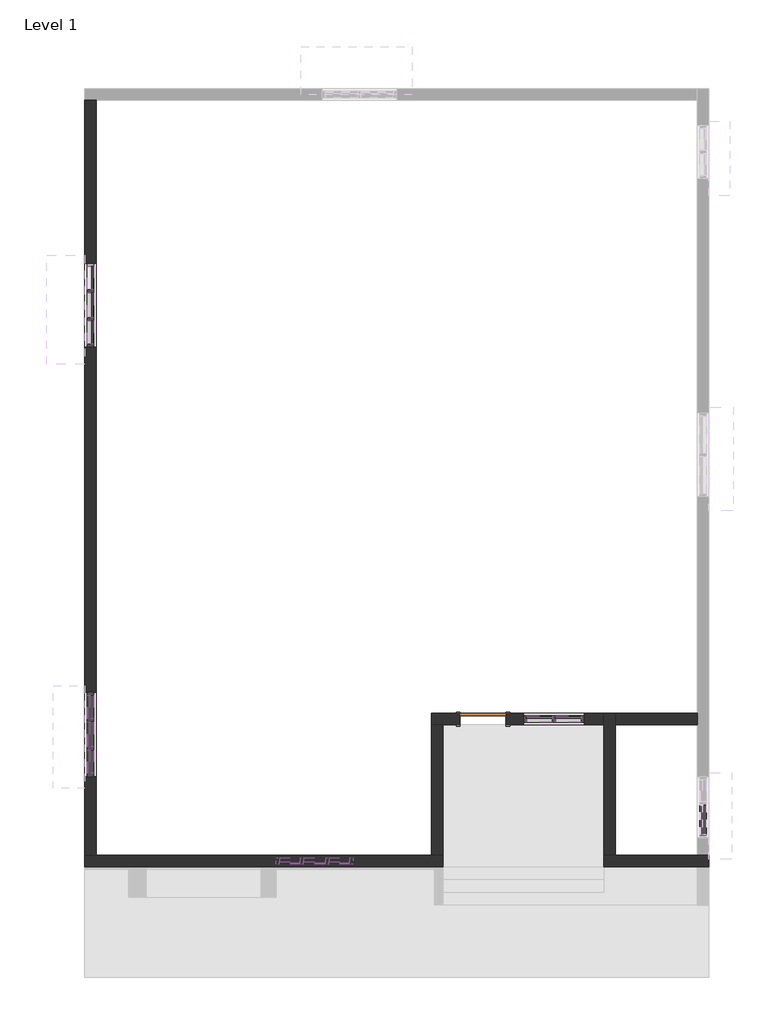
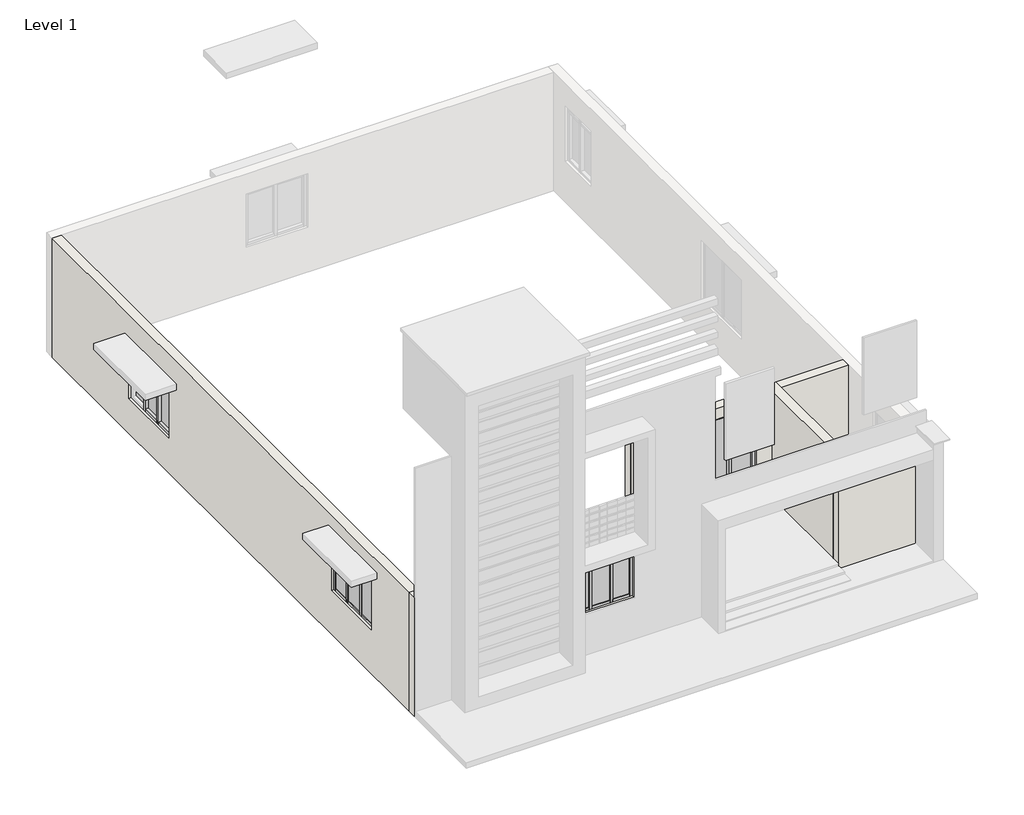
# One storey, part 1 of 2: 36 members, 11 plates, 7 walls, 1 door.
"""IFC4 building model written with IfcOpenShell, lengths in millimetres."""

from ifc_helpers import new_model, si_unit, frame, origin, origin_with_axes, place, context, project, spatial, polyline, outline, extrude, faceted_brep, transform, mapped, element, save
from components import door_0ca8825f, member_bc7dbe04, member_dc106669, member_d01054ea, member_be902966, member_0b7646a3, member_e710c4d8, member_6a3d3fef, member_e5d39754, member_2ebf4a73, member_5535eeb3, member_4b9f21bc, member_b02ddeff, member_347b2a6f, member_041bc147, system_panel_glazed_6aba1888, system_panel_glazed_fa064951, system_panel_glazed_b01bb026, system_panel_glazed_b47451c9, system_panel_glazed_f8dc496e, system_panel_glazed_bdc4a67b, system_panel_glazed_464a4b5e

model = new_model("IFC4")

# Units and contexts
model_context = context("Model", 3, world=origin())
ifc_project = project(units=[si_unit("LENGTHUNIT", "METRE", prefix="MILLI")], contexts=[model_context])

# Site, building, storey
site = spatial("IfcSite", under=ifc_project)
building = spatial("IfcBuilding", under=site)
storey = spatial("IfcBuildingStorey", under=building, Name="Level 1", Elevation=0.0)

# Door
placement = place(None, origin())
door_shape = door_0ca8825f(model_context)
element("IfcDoor", 1, ObjectType="Single-Flush : 36\" x 84\"", at=placement, inside=storey, context=model_context, shape_type="MappedRepresentation", body=[
    mapped(door_shape, transform((-8298.2859258, -8867.3777232, 0.0), x_axis=(1.0, 0.0, 0.0), y_axis=(0.0, 1.0, 0.0), z_axis=(0.0, 0.0, 1.0))),
])

# Members
member_shape = member_bc7dbe04(model_context)
element("IfcMember", 2, ObjectType="Rectangular Mullion : 2.5\" x 5\" rectangular", at=placement, inside=storey, context=model_context, shape_type="MappedRepresentation", body=[
    mapped(member_shape, transform((-11428.8359258, -11686.7777232, 1204.6732896), x_axis=(0.0, 0.0, -1.0), y_axis=(0.0, 1.0, 0.0), z_axis=(1.0, 0.0, 0.0))),
])
member_2_shape = member_dc106669(model_context)
element("IfcMember", 3, ObjectType="Rectangular Mullion : 2.5\" x 5\" rectangular", at=placement, inside=storey, context=model_context, shape_type="MappedRepresentation", body=[
    mapped(member_2_shape, transform((-11936.8359258, -11686.7777232, 1204.6732896), x_axis=(0.0, 0.0, -1.0), y_axis=(0.0, 1.0, 0.0), z_axis=(1.0, 0.0, 0.0))),
])
element("IfcMember", 4, ObjectType="Rectangular Mullion : 2.5\" x 5\" rectangular", at=placement, inside=storey, context=model_context, shape_type="MappedRepresentation", body=[
    mapped(member_2_shape, transform((-10952.5859258, -11686.7777232, 1204.6732896), x_axis=(0.0, 0.0, -1.0), y_axis=(0.0, 1.0, 0.0), z_axis=(1.0, 0.0, 0.0))),
])
member_3_shape = member_d01054ea(model_context)
element("IfcMember", 5, ObjectType="Rectangular Mullion : 2.5\" x 5\" rectangular", at=placement, inside=storey, context=model_context, shape_type="MappedRepresentation", body=[
    mapped(member_3_shape, transform((-11905.0859258, -11686.7777232, 1204.6732896), x_axis=(-1.0, 0.0, 0.0), y_axis=(0.0, 1.0, 0.0), z_axis=(0.0, 0.0, -1.0))),
])
element("IfcMember", 6, ObjectType="Rectangular Mullion : 2.5\" x 5\" rectangular", at=placement, inside=storey, context=model_context, shape_type="MappedRepresentation", body=[
    mapped(member_3_shape, transform((-11397.0859258, -11686.7777232, 1204.6732896), x_axis=(-1.0, 0.0, 0.0), y_axis=(0.0, 1.0, 0.0), z_axis=(0.0, 0.0, -1.0))),
])
element("IfcMember", 7, ObjectType="Rectangular Mullion : 2.5\" x 5\" rectangular", at=placement, inside=storey, context=model_context, shape_type="MappedRepresentation", body=[
    mapped(member_2_shape, transform((-11365.3359258, -11686.7777232, 2726.819022), x_axis=(0.0, 0.0, 1.0), y_axis=(0.0, 1.0, 0.0), z_axis=(-1.0, 0.0, 0.0))),
])
element("IfcMember", 8, ObjectType="Rectangular Mullion : 2.5\" x 5\" rectangular", at=placement, inside=storey, context=model_context, shape_type="MappedRepresentation", body=[
    mapped(member_2_shape, transform((-12349.5859258, -11686.7777232, 2726.819022), x_axis=(0.0, 0.0, 1.0), y_axis=(0.0, 1.0, 0.0), z_axis=(-1.0, 0.0, 0.0))),
])
element("IfcMember", 9, ObjectType="Rectangular Mullion : 2.5\" x 5\" rectangular", at=placement, inside=storey, context=model_context, shape_type="MappedRepresentation", body=[
    mapped(member_shape, transform((-11873.3359258, -11686.7777232, 2726.819022), x_axis=(0.0, 0.0, 1.0), y_axis=(0.0, 1.0, 0.0), z_axis=(-1.0, 0.0, 0.0))),
])
member_4_shape = member_be902966(model_context)
element("IfcMember", 10, ObjectType="Rectangular Mullion : 2.5\" x 5\" rectangular", at=placement, inside=storey, context=model_context, shape_type="MappedRepresentation", body=[
    mapped(member_4_shape, transform((-12413.0859258, -11686.7777232, 1204.6732896), x_axis=(-1.0, 0.0, 0.0), y_axis=(0.0, 1.0, 0.0), z_axis=(0.0, 0.0, -1.0))),
])
element("IfcMember", 11, ObjectType="Rectangular Mullion : 2.5\" x 5\" rectangular", at=placement, inside=storey, context=model_context, shape_type="MappedRepresentation", body=[
    mapped(member_4_shape, transform((-10889.0859258, -11686.7777232, 2726.819022), x_axis=(1.0, 0.0, 0.0), y_axis=(0.0, 1.0, 0.0), z_axis=(0.0, 0.0, 1.0))),
])
member_5_shape = member_0b7646a3(model_context)
element("IfcMember", 12, ObjectType="Rectangular Mullion : 2.5\" x 5\" rectangular", at=placement, inside=storey, context=model_context, shape_type="MappedRepresentation", body=[
    mapped(member_5_shape, transform((-6920.3359258, -8867.3777232, 2781.5010692), x_axis=(0.0, 0.0, 1.0), y_axis=(0.0, -1.0, 0.0), z_axis=(1.0, 0.0, 0.0))),
])
element("IfcMember", 13, ObjectType="Rectangular Mullion : 2.5\" x 5\" rectangular", at=placement, inside=storey, context=model_context, shape_type="MappedRepresentation", body=[
    mapped(member_5_shape, transform((-6342.4859258, -8867.3777232, 2781.5010692), x_axis=(0.0, 0.0, 1.0), y_axis=(0.0, -1.0, 0.0), z_axis=(1.0, 0.0, 0.0))),
])
member_6_shape = member_e710c4d8(model_context)
element("IfcMember", 14, ObjectType="Rectangular Mullion : 2.5\" x 5\" rectangular", at=placement, inside=storey, context=model_context, shape_type="MappedRepresentation", body=[
    mapped(member_6_shape, transform((-6888.5859258, -8867.3777232, 1004.1703665), x_axis=(1.0, 0.0, 0.0), y_axis=(0.0, -1.0, 0.0), z_axis=(0.0, 0.0, -1.0))),
])
element("IfcMember", 15, ObjectType="Rectangular Mullion : 2.5\" x 5\" rectangular", at=placement, inside=storey, context=model_context, shape_type="MappedRepresentation", body=[
    mapped(member_5_shape, transform((-6856.8359258, -8867.3777232, 1004.1703665), x_axis=(0.0, 0.0, -1.0), y_axis=(0.0, -1.0, 0.0), z_axis=(-1.0, 0.0, 0.0))),
])
element("IfcMember", 16, ObjectType="Rectangular Mullion : 2.5\" x 5\" rectangular", at=placement, inside=storey, context=model_context, shape_type="MappedRepresentation", body=[
    mapped(member_5_shape, transform((-7434.6859258, -8867.3777232, 1004.1703665), x_axis=(0.0, 0.0, -1.0), y_axis=(0.0, -1.0, 0.0), z_axis=(-1.0, 0.0, 0.0))),
])
member_7_shape = member_6a3d3fef(model_context)
element("IfcMember", 17, ObjectType="Rectangular Mullion : 2.5\" x 5\" rectangular", at=placement, inside=storey, context=model_context, shape_type="MappedRepresentation", body=[
    mapped(member_7_shape, transform((-7498.1859258, -8867.3777232, 2781.5010692), x_axis=(-1.0, 0.0, 0.0), y_axis=(0.0, -1.0, 0.0), z_axis=(0.0, 0.0, 1.0))),
])
element("IfcMember", 18, ObjectType="Rectangular Mullion : 2.5\" x 5\" rectangular", at=placement, inside=storey, context=model_context, shape_type="MappedRepresentation", body=[
    mapped(member_7_shape, transform((-6278.9859258, -8867.3777232, 1004.1703665), x_axis=(1.0, 0.0, 0.0), y_axis=(0.0, -1.0, 0.0), z_axis=(0.0, 0.0, -1.0))),
])
member_8_shape = member_e5d39754(model_context)
element("IfcMember", 19, ObjectType="Rectangular Mullion : 2.5\" x 5\" rectangular", at=placement, inside=storey, context=model_context, shape_type="MappedRepresentation", body=[
    mapped(member_8_shape, transform((-3916.7859258, -11166.0777232, 1144.0804944), x_axis=(0.0, 0.0, -1.0), y_axis=(1.0, 0.0, 0.0), z_axis=(0.0, -1.0, 0.0))),
])
member_9_shape = member_2ebf4a73(model_context)
element("IfcMember", 20, ObjectType="Rectangular Mullion : 2.5\" x 5\" rectangular", at=placement, inside=storey, context=model_context, shape_type="MappedRepresentation", body=[
    mapped(member_9_shape, transform((-16108.7859258, -8924.5277232, 2585.6396252), x_axis=(0.0, 0.0, 1.0), y_axis=(1.0, 0.0, 0.0), z_axis=(0.0, 1.0, 0.0))),
])
element("IfcMember", 21, ObjectType="Rectangular Mullion : 2.5\" x 5\" rectangular", at=placement, inside=storey, context=model_context, shape_type="MappedRepresentation", body=[
    mapped(member_9_shape, transform((-16108.7859258, -885.4277232, 2325.7757409), x_axis=(0.0, 0.0, 1.0), y_axis=(-1.0, 0.0, 0.0), z_axis=(0.0, -1.0, 0.0))),
])
member_10_shape = member_5535eeb3(model_context)
element("IfcMember", 22, ObjectType="Rectangular Mullion : 2.5\" x 5\" rectangular", at=placement, inside=storey, context=model_context, shape_type="MappedRepresentation", body=[
    mapped(member_10_shape, transform((-16108.7859258, -9483.3277232, 2585.6396252), x_axis=(0.0, 0.0, 1.0), y_axis=(1.0, 0.0, 0.0), z_axis=(0.0, 1.0, 0.0))),
])
element("IfcMember", 23, ObjectType="Rectangular Mullion : 2.5\" x 5\" rectangular", at=placement, inside=storey, context=model_context, shape_type="MappedRepresentation", body=[
    mapped(member_10_shape, transform((-16108.7859258, -8397.4777232, 2585.6396252), x_axis=(0.0, 0.0, 1.0), y_axis=(1.0, 0.0, 0.0), z_axis=(0.0, 1.0, 0.0))),
])
element("IfcMember", 24, ObjectType="Rectangular Mullion : 2.5\" x 5\" rectangular", at=placement, inside=storey, context=model_context, shape_type="MappedRepresentation", body=[
    mapped(member_10_shape, transform((-16108.7859258, -326.6277232, 2325.7757409), x_axis=(0.0, 0.0, 1.0), y_axis=(-1.0, 0.0, 0.0), z_axis=(0.0, -1.0, 0.0))),
])
element("IfcMember", 25, ObjectType="Rectangular Mullion : 2.5\" x 5\" rectangular", at=placement, inside=storey, context=model_context, shape_type="MappedRepresentation", body=[
    mapped(member_10_shape, transform((-16108.7859258, -1412.4777232, 2325.7757409), x_axis=(0.0, 0.0, 1.0), y_axis=(-1.0, 0.0, 0.0), z_axis=(0.0, -1.0, 0.0))),
])
member_11_shape = member_4b9f21bc(model_context)
element("IfcMember", 26, ObjectType="Rectangular Mullion : 2.5\" x 5\" rectangular", at=placement, inside=storey, context=model_context, shape_type="MappedRepresentation", body=[
    mapped(member_11_shape, transform((-16108.7859258, -8892.7777232, 1138.697398), x_axis=(0.0, 1.0, 0.0), y_axis=(1.0, 0.0, 0.0), z_axis=(0.0, 0.0, -1.0))),
])
element("IfcMember", 27, ObjectType="Rectangular Mullion : 2.5\" x 5\" rectangular", at=placement, inside=storey, context=model_context, shape_type="MappedRepresentation", body=[
    mapped(member_11_shape, transform((-16108.7859258, -9451.5777232, 1138.697398), x_axis=(0.0, 1.0, 0.0), y_axis=(1.0, 0.0, 0.0), z_axis=(0.0, 0.0, -1.0))),
])
element("IfcMember", 28, ObjectType="Rectangular Mullion : 2.5\" x 5\" rectangular", at=placement, inside=storey, context=model_context, shape_type="MappedRepresentation", body=[
    mapped(member_9_shape, transform((-16108.7859258, -9419.8277232, 1138.697398), x_axis=(0.0, 0.0, -1.0), y_axis=(1.0, 0.0, 0.0), z_axis=(0.0, -1.0, 0.0))),
])
element("IfcMember", 29, ObjectType="Rectangular Mullion : 2.5\" x 5\" rectangular", at=placement, inside=storey, context=model_context, shape_type="MappedRepresentation", body=[
    mapped(member_9_shape, transform((-16108.7859258, -390.1277232, 897.5231842), x_axis=(0.0, 0.0, -1.0), y_axis=(-1.0, 0.0, 0.0), z_axis=(0.0, 1.0, 0.0))),
])
element("IfcMember", 30, ObjectType="Rectangular Mullion : 2.5\" x 5\" rectangular", at=placement, inside=storey, context=model_context, shape_type="MappedRepresentation", body=[
    mapped(member_10_shape, transform((-16108.7859258, -8861.0277232, 1138.697398), x_axis=(0.0, 0.0, -1.0), y_axis=(1.0, 0.0, 0.0), z_axis=(0.0, -1.0, 0.0))),
])
element("IfcMember", 31, ObjectType="Rectangular Mullion : 2.5\" x 5\" rectangular", at=placement, inside=storey, context=model_context, shape_type="MappedRepresentation", body=[
    mapped(member_10_shape, transform((-16108.7859258, -9946.8777232, 1138.697398), x_axis=(0.0, 0.0, -1.0), y_axis=(1.0, 0.0, 0.0), z_axis=(0.0, -1.0, 0.0))),
])
element("IfcMember", 32, ObjectType="Rectangular Mullion : 2.5\" x 5\" rectangular", at=placement, inside=storey, context=model_context, shape_type="MappedRepresentation", body=[
    mapped(member_10_shape, transform((-16108.7859258, -948.9277232, 897.5231842), x_axis=(0.0, 0.0, -1.0), y_axis=(-1.0, 0.0, 0.0), z_axis=(0.0, 1.0, 0.0))),
])
member_12_shape = member_b02ddeff(model_context)
element("IfcMember", 33, ObjectType="Rectangular Mullion : 2.5\" x 5\" rectangular", at=placement, inside=storey, context=model_context, shape_type="MappedRepresentation", body=[
    mapped(member_12_shape, transform((-16108.7859258, -8333.9777232, 1138.697398), x_axis=(0.0, 1.0, 0.0), y_axis=(1.0, 0.0, 0.0), z_axis=(0.0, 0.0, -1.0))),
])
element("IfcMember", 34, ObjectType="Rectangular Mullion : 2.5\" x 5\" rectangular", at=placement, inside=storey, context=model_context, shape_type="MappedRepresentation", body=[
    mapped(member_12_shape, transform((-16108.7859258, -10010.3777232, 2585.6396252), x_axis=(0.0, -1.0, 0.0), y_axis=(1.0, 0.0, 0.0), z_axis=(0.0, 0.0, 1.0))),
])
member_13_shape = member_347b2a6f(model_context)
element("IfcMember", 35, ObjectType="Rectangular Mullion : 2.5\" x 5\" rectangular", at=placement, inside=storey, context=model_context, shape_type="MappedRepresentation", body=[
    mapped(member_13_shape, transform((-16108.7859258, -358.3777232, 897.5231842), x_axis=(0.0, -1.0, 0.0), y_axis=(-1.0, 0.0, 0.0), z_axis=(0.0, 0.0, -1.0))),
])
element("IfcMember", 36, ObjectType="Rectangular Mullion : 2.5\" x 5\" rectangular", at=placement, inside=storey, context=model_context, shape_type="MappedRepresentation", body=[
    mapped(member_13_shape, transform((-16108.7859258, -917.1777232, 897.5231842), x_axis=(0.0, -1.0, 0.0), y_axis=(-1.0, 0.0, 0.0), z_axis=(0.0, 0.0, -1.0))),
])
member_14_shape = member_041bc147(model_context)
element("IfcMember", 37, ObjectType="Rectangular Mullion : 2.5\" x 5\" rectangular", at=placement, inside=storey, context=model_context, shape_type="MappedRepresentation", body=[
    mapped(member_14_shape, transform((-16108.7859258, -1475.9777232, 897.5231842), x_axis=(0.0, -1.0, 0.0), y_axis=(-1.0, 0.0, 0.0), z_axis=(0.0, 0.0, -1.0))),
])

# Plates
system_panel_glazed_shape = system_panel_glazed_6aba1888(model_context)
element("IfcPlate", 38, ObjectType="System Panel : Glazed", at=placement, inside=storey, context=model_context, shape_type="MappedRepresentation", body=[
    mapped(system_panel_glazed_shape, transform((-11158.9609258, -11686.7777232, 1268.1732896), x_axis=(-1.0, 0.0, 0.0), y_axis=(0.0, -1.0, 0.0), z_axis=(0.0, 0.0, 1.0))),
])
element("IfcPlate", 39, ObjectType="System Panel : Glazed", at=placement, inside=storey, context=model_context, shape_type="MappedRepresentation", body=[
    mapped(system_panel_glazed_shape, transform((-12143.2109258, -11686.7777232, 1268.1732896), x_axis=(-1.0, 0.0, 0.0), y_axis=(0.0, -1.0, 0.0), z_axis=(0.0, 0.0, 1.0))),
])
system_panel_glazed_2_shape = system_panel_glazed_fa064951(model_context)
element("IfcPlate", 40, ObjectType="System Panel : Glazed", at=placement, inside=storey, context=model_context, shape_type="MappedRepresentation", body=[
    mapped(system_panel_glazed_2_shape, transform((-11651.0859258, -11686.7777232, 1268.1732896), x_axis=(-1.0, 0.0, 0.0), y_axis=(0.0, -1.0, 0.0), z_axis=(0.0, 0.0, 1.0))),
])
system_panel_glazed_3_shape = system_panel_glazed_b01bb026(model_context)
element("IfcPlate", 41, ObjectType="System Panel : Glazed", at=placement, inside=storey, context=model_context, shape_type="MappedRepresentation", body=[
    mapped(system_panel_glazed_3_shape, transform((-7177.5109258, -8867.3777232, 1067.6703665), x_axis=(1.0, 0.0, 0.0), y_axis=(0.0, 1.0, 0.0), z_axis=(0.0, 0.0, 1.0))),
])
element("IfcPlate", 42, ObjectType="System Panel : Glazed", at=placement, inside=storey, context=model_context, shape_type="MappedRepresentation", body=[
    mapped(system_panel_glazed_3_shape, transform((-6599.6609258, -8867.3777232, 1067.6703665), x_axis=(1.0, 0.0, 0.0), y_axis=(0.0, 1.0, 0.0), z_axis=(0.0, 0.0, 1.0))),
])
system_panel_glazed_4_shape = system_panel_glazed_b47451c9(model_context)
element("IfcPlate", 43, ObjectType="System Panel : Glazed", at=placement, inside=storey, context=model_context, shape_type="MappedRepresentation", body=[
    mapped(system_panel_glazed_4_shape, transform((-16108.7859258, -9715.1027232, 1202.197398), x_axis=(0.0, 1.0, 0.0), y_axis=(-1.0, 0.0, 0.0), z_axis=(0.0, 0.0, 1.0))),
])
element("IfcPlate", 44, ObjectType="System Panel : Glazed", at=placement, inside=storey, context=model_context, shape_type="MappedRepresentation", body=[
    mapped(system_panel_glazed_4_shape, transform((-16108.7859258, -8629.2527232, 1202.197398), x_axis=(0.0, 1.0, 0.0), y_axis=(-1.0, 0.0, 0.0), z_axis=(0.0, 0.0, 1.0))),
])
system_panel_glazed_5_shape = system_panel_glazed_f8dc496e(model_context)
element("IfcPlate", 45, ObjectType="System Panel : Glazed", at=placement, inside=storey, context=model_context, shape_type="MappedRepresentation", body=[
    mapped(system_panel_glazed_5_shape, transform((-16108.7859258, -9172.1777232, 1202.197398), x_axis=(0.0, 1.0, 0.0), y_axis=(-1.0, 0.0, 0.0), z_axis=(0.0, 0.0, 1.0))),
])
system_panel_glazed_6_shape = system_panel_glazed_bdc4a67b(model_context)
element("IfcPlate", 46, ObjectType="System Panel : Glazed", at=placement, inside=storey, context=model_context, shape_type="MappedRepresentation", body=[
    mapped(system_panel_glazed_6_shape, transform((-16108.7859258, -94.8527232, 961.0231842), x_axis=(0.0, -1.0, 0.0), y_axis=(1.0, 0.0, 0.0), z_axis=(0.0, 0.0, 1.0))),
])
element("IfcPlate", 47, ObjectType="System Panel : Glazed", at=placement, inside=storey, context=model_context, shape_type="MappedRepresentation", body=[
    mapped(system_panel_glazed_6_shape, transform((-16108.7859258, -1180.7027232, 961.0231842), x_axis=(0.0, -1.0, 0.0), y_axis=(1.0, 0.0, 0.0), z_axis=(0.0, 0.0, 1.0))),
])
system_panel_glazed_7_shape = system_panel_glazed_464a4b5e(model_context)
element("IfcPlate", 48, ObjectType="System Panel : Glazed", at=placement, inside=storey, context=model_context, shape_type="MappedRepresentation", body=[
    mapped(system_panel_glazed_7_shape, transform((-16108.7859258, -637.7777232, 961.0231842), x_axis=(0.0, -1.0, 0.0), y_axis=(1.0, 0.0, 0.0), z_axis=(0.0, 0.0, 1.0))),
])

# Walls
element("IfcWall", 49, ObjectType="9\"", at=placement, inside=storey, context=model_context, shape_type="Brep", body=[
    faceted_brep([(-16223.0859258, -11801.0777232, 0.0), (-9098.3859258, -11801.0777232, 0.0), (-9098.3859258, -11801.0777232, 3048.0), (-16223.0859258, -11801.0777232, 3048.0), (-10889.0859258, -11801.0777232, 2726.819022), (-10889.0859258, -11801.0777232, 1204.6732896), (-12413.0859258, -11801.0777232, 1204.6732896), (-12413.0859258, -11801.0777232, 2726.819022), (-9098.3859258, -11572.4777232, 0.0), (-9326.9859258, -11572.4777232, 0.0), (-15994.4859258, -11572.4777232, 0.0), (-16223.0859258, -11572.4777232, 0.0), (-16223.0859258, -11572.4777232, 3048.0), (-15994.4859258, -11572.4777232, 3048.0), (-9326.9859258, -11572.4777232, 3048.0), (-9098.3859258, -11572.4777232, 3048.0), (-10889.0859258, -11572.4777232, 1204.6732896), (-10889.0859258, -11572.4777232, 2726.819022), (-12413.0859258, -11572.4777232, 2726.819022), (-12413.0859258, -11572.4777232, 1204.6732896)], [[[0, 1, 2, 3], [4, 5, 6, 7]], [[8, 9, 10, 11, 12, 13, 14, 15], [16, 17, 18, 19]], [[1, 0, 11, 10, 9, 8]], [[2, 1, 8, 15]], [[3, 2, 15, 14, 13, 12]], [[0, 3, 12, 11]], [[16, 5, 4, 17]], [[17, 4, 7, 18]], [[18, 7, 6, 19]], [[5, 16, 19, 6]]]),
])
element("IfcWall", 50, ObjectType="9\"", at=placement, inside=storey, context=model_context, shape_type="SweptSolid", body=[
    extrude(outline(polyline([(3438.9222768, 0.0), (-11572.4777232, 0.0), (-11572.4777232, 3048.0), (3438.9222768, 3048.0), (3438.9222768, 0.0)]), holes=[polyline([(-10010.3777232, 2585.6396252), (-10010.3777232, 1138.697398), (-8333.9777232, 1138.697398), (-8333.9777232, 2585.6396252), (-10010.3777232, 2585.6396252)]), polyline([(200.4222768, 897.5231842), (200.4222768, 2325.7757409), (-1475.9777232, 2325.7757409), (-1475.9777232, 897.5231842), (200.4222768, 897.5231842)])]), frame((-16223.0859258, 0.0, 0.0), z_axis=(1.0, 0.0, 0.0), x_axis=(0.0, 1.0, 0.0)), (0.0, 0.0, 1.0), 228.6),
])
element("IfcWall", 51, ObjectType="9\"", at=placement, inside=storey, context=model_context, shape_type="Brep", body=[
    faceted_brep([(-5669.3859258, -11572.4777232, 0.0), (-5669.3859258, -8981.6777232, 0.0), (-5669.3859258, -8753.0777232, 0.0), (-5669.3859258, -8753.0777232, 3048.0), (-5669.3859258, -8981.6777232, 3048.0), (-5669.3859258, -11572.4777232, 3048.0), (-5897.9859258, -11572.4777232, 0.0), (-5897.9859258, -11572.4777232, 3048.0), (-5897.9859258, -8981.6777232, 3048.0), (-5897.9859258, -8753.0777232, 3048.0), (-5897.9859258, -8753.0777232, 0.0), (-5897.9859258, -8981.6777232, 0.0)], [[[0, 1, 2, 3, 4, 5]], [[6, 7, 8, 9, 10, 11]], [[2, 1, 0, 6, 11, 10]], [[5, 4, 3, 9, 8, 7]], [[0, 5, 7, 6]], [[3, 2, 10, 9]]]),
])
element("IfcWall", 52, ObjectType="9\"", at=placement, inside=storey, context=model_context, shape_type="Brep", body=[
    faceted_brep([(-9326.9859258, -8753.0777232, 3048.0), (-5897.9859258, -8753.0777232, 3048.0), (-5897.9859258, -8753.0777232, 0.0), (-7841.0859258, -8753.0777232, 0.0), (-7841.0859258, -8753.0777232, 2133.6), (-8755.4859258, -8753.0777232, 2133.6), (-8755.4859258, -8753.0777232, 0.0), (-9326.9859258, -8753.0777232, 0.0), (-7498.1859258, -8753.0777232, 2781.5010692), (-7498.1859258, -8753.0777232, 1004.1703665), (-6278.9859258, -8753.0777232, 1004.1703665), (-6278.9859258, -8753.0777232, 2781.5010692), (-5897.9859258, -8981.6777232, 3048.0), (-9098.3859258, -8981.6777232, 3048.0), (-9326.9859258, -8981.6777232, 3048.0), (-9326.9859258, -8981.6777232, 0.0), (-9098.3859258, -8981.6777232, 0.0), (-8755.4859258, -8981.6777232, 0.0), (-8755.4859258, -8981.6777232, 2133.6), (-7841.0859258, -8981.6777232, 2133.6), (-7841.0859258, -8981.6777232, 0.0), (-5897.9859258, -8981.6777232, 0.0), (-7498.1859258, -8981.6777232, 1004.1703665), (-7498.1859258, -8981.6777232, 2781.5010692), (-6278.9859258, -8981.6777232, 2781.5010692), (-6278.9859258, -8981.6777232, 1004.1703665)], [[[0, 1, 2, 3, 4, 5, 6, 7], [8, 9, 10, 11]], [[12, 13, 14, 15, 16, 17, 18, 19, 20, 21], [22, 23, 24, 25]], [[2, 21, 20, 3]], [[15, 7, 6, 17, 16]], [[1, 0, 14, 13, 12]], [[2, 1, 12, 21]], [[0, 7, 15, 14]], [[4, 3, 20, 19]], [[5, 4, 19, 18]], [[6, 5, 18, 17]], [[22, 9, 8, 23]], [[23, 8, 11, 24]], [[24, 11, 10, 25]], [[9, 22, 25, 10]]]),
])
element("IfcWall", 53, ObjectType="9\"", at=placement, inside=storey, context=model_context, shape_type="SweptSolid", body=[
    extrude(outline(polyline([(-9326.9859258, -11572.4777232), (-9326.9859258, -8981.6777232), (-9098.3859258, -8981.6777232), (-9098.3859258, -11572.4777232), (-9326.9859258, -11572.4777232)])), origin_with_axes(), (0.0, 0.0, 1.0), 3048.0),
])
element("IfcWall", 54, ObjectType="9\"", at=placement, inside=storey, context=model_context, shape_type="SweptSolid", body=[
    extrude(outline(polyline([(-4031.0859258, -8981.6777232), (-5669.3859258, -8981.6777232), (-5669.3859258, -8753.0777232), (-4031.0859258, -8753.0777232), (-4031.0859258, -8981.6777232)])), origin_with_axes(), (0.0, 0.0, 1.0), 3048.0),
])
element("IfcWall", 55, ObjectType="9\"", at=placement, inside=storey, context=model_context, shape_type="Brep", body=[
    faceted_brep([(-5897.9859258, -11801.0777232, 0.0), (-3802.4859258, -11801.0777232, 0.0), (-3802.4859258, -11801.0777232, 3048.0), (-5897.9859258, -11801.0777232, 3048.0), (-5897.9859258, -11572.4777232, 0.0), (-5897.9859258, -11572.4777232, 3048.0), (-5669.3859258, -11572.4777232, 3048.0), (-4031.0859258, -11572.4777232, 3048.0), (-3802.4859258, -11572.4777232, 3048.0), (-3802.4859258, -11572.4777232, 0.0), (-4031.0859258, -11572.4777232, 0.0), (-5669.3859258, -11572.4777232, 0.0)], [[[0, 1, 2, 3]], [[4, 5, 6, 7, 8, 9, 10, 11]], [[1, 0, 4, 11, 10, 9]], [[3, 2, 8, 7, 6, 5]], [[0, 3, 5, 4]], [[2, 1, 9, 8]]]),
])

save(model, "model.ifc")

# Revit data of these elements
# Type "Single-Flush : 36\" x 84\""
#   Type Mark = "1"
#   Construction Type Id = "MDOOR"
#   Assembly Code = "C1020"
#   Analytic Construction = "Metal"
#   Thickness = 0' - 2"
#   Heat Transfer Coefficient (U) = 0.651978 BTU/(h·ft²·°F)
#   Height = 7' - 0"
#   Trim Projection Ext = 0' - 1"
#   Trim Projection Int = 0' - 1"
#   Trim Width = 0' - 3"
#   Width = 3' - 0"
#   Define Thermal Properties by = 1
#   Define Thermal Properties by = 1
#   Door Material = Door - Panel
#   Frame Material = Door - Frame
#   Visual Light Transmittance = 0
#   Solar Heat Gain Coefficient = 0
#   Function = (empty or 0)
#   Wall Closure = (empty or 0)
# Type "Rectangular Mullion : 2.5\" x 5\" rectangular"
#   built-in parameter 1007304 = 0.416667 (stored number, unit not read)
#   built-in parameter 1007301 = 0.104167 (stored number, unit not read)
#   built-in parameter 1007300 = 0.104167 (stored number, unit not read)
# Type "System Panel : Glazed"
#   Construction Type Id = "GSP4R"
#   Analytic Construction = "1/8 in Pilkington single glazing"
#   Visual Light Transmittance = 0.9
#   Solar Heat Gain Coefficient = 0.86
#   Heat Transfer Coefficient (U) = 1.18115 BTU/(h·ft²·°F)
#   Define Thermal Properties by = 1
# Type "9\""
#   Assembly Code = "B2010"
#   Layers, outside or top first: 0' - 9" no material (function 1)
# Element 1 (IfcDoor, "Single-Flush : 36\" x 84\"")
#   Phase Created = New Construction
#   Materials on its faces: "Door - Frame", "Door - Panel"
# Elements 2, 3, 4, 5, 6, 7, 8, 9, 10, 11, 12, 13, 14, 15, 16, 17, 18, 19, 20, 21, 22, 23, 24, 25, 26, 27, 28, 29, 30, 31, 32, 33, 34, 35, 36, 37 (IfcMember, "Rectangular Mullion : 2.5\" x 5\" rectangular")
#   Phase Created = New Construction
#   Materials on its faces: "Aluminum"
# Elements 38, 39, 40, 41, 42, 43, 44, 45, 46, 47, 48 (IfcPlate, "System Panel : Glazed")
#   Phase Created = New Construction
#   Materials on its faces: "Glass"
# Elements 49, 50, 51, 52, 53, 54, 55 (IfcWall, "9\"")
#   Top Offset = 0' - 0"
#   Base Offset = 0' - 0"
#   Unconnected Height = 10' - 0"
#   wall height = 10' - 0"
#   Phase Created = New Construction
#   Base Constraint = Level 1
#   Materials on its faces: "Default Wall"
# Materials
#   "Door - Panel": class "Wood", colour RGB 210 159 95, transparency 0, Cost = 0
#   "Door - Frame": colour RGB 118 70 51, transparency 0, Cost = 0
#   "Aluminum": class "Metal", colour RGB 247 247 247, transparency 0, Description = "Aluminum 6061", Cost = 0
#   "Glass": class "Glass", colour RGB 0 128 192, transparency 0.75, Description = "Soda Lime Glass", Cost = 0
#   "Default Wall": colour RGB 128 128 128, transparency 0, Cost = 0
